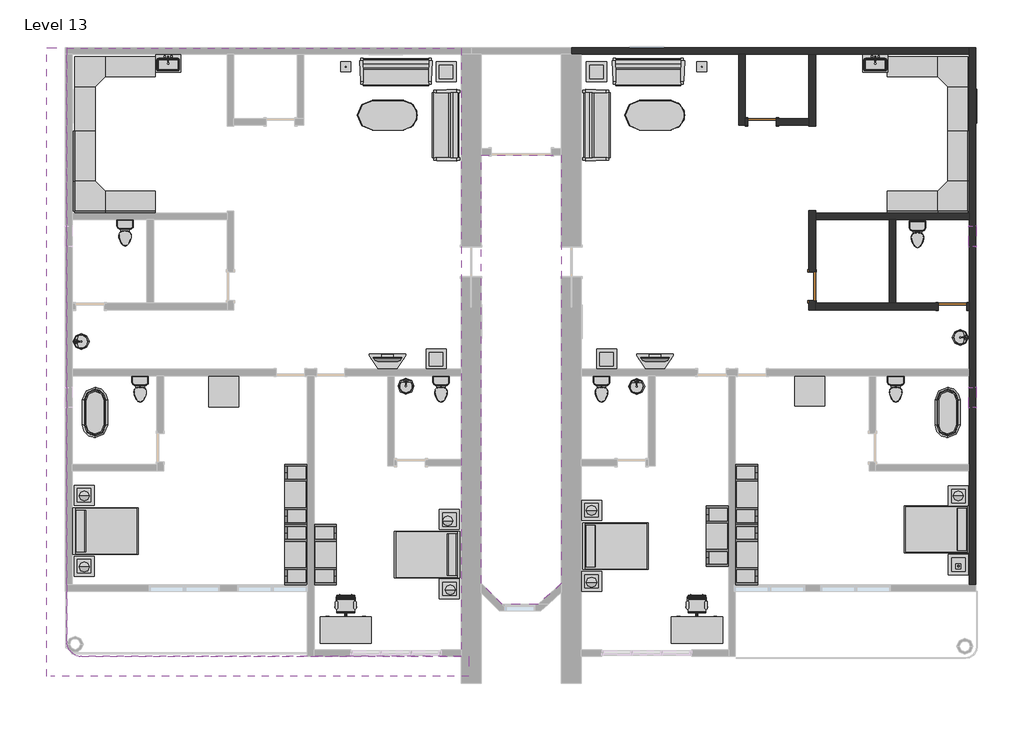
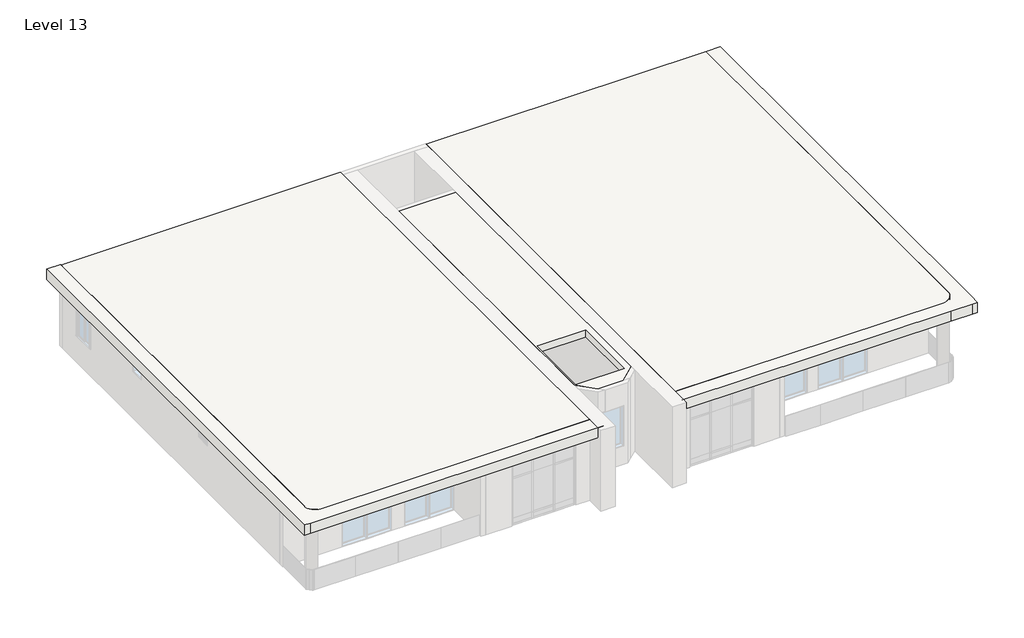
# One storey, part 3 of 3: 42 furniture elements, 14 flow terminals, 10 light fixtures, 9 walls, 3 doors, 3 slabs, 3 windows.
# Revit data of these elements (continued)
# Elements 38, 39 (IfcFurniture, "TV - Flat Screen : 32\"")
#   Stand = yes
#   Phase Created = New Construction
#   Materials on its faces: "TV - Black", "TV - Glass", "TV - Screen"
# Elements 40, 41 (IfcFurniture, "TV Stand : TV Stand")
#   Phase Created = New Construction
#   Materials on its faces: "Melamine - Gray", "Glass - Shelves"
# Elements 42, 43, 44, 45, 46, 47, 48, 49, 50, 51, 52, 53 (IfcFurniture, "Table-Coffee : 24\" x 24\" x 24\"")
#   Phase Created = New Construction
#   Materials on its faces: "Glass - Clear, Grey"
# Elements 54, 55 (IfcFurniture, "Table-Dining Oval : 36\" x 72\"")
#   Phase Created = New Construction
#   Materials on its faces: "Steel, Chrome Plated", "Glass - Clear, Grey"
# Elements 56, 57 (IfcFurniture, "Table-Rectangular : 36\" x 36\"")
#   Phase Created = New Construction
#   Materials on its faces: "Birch"
# Elements 58, 59 (IfcFurniture, "Work Station Cubicle : 96\" x 96\"")
#   Phase Created = New Construction
#   Materials on its faces: "Textile - Light Gray", "Laminate, Ivory, Matte"
# Element 60 (IfcLightFixture, "100W - 120V")
#   Mark = "144"
#   Phase Created = New Construction
#   Materials on its faces: "Steel, Chrome Plated", "Glass, Frosted"
# Element 61 (IfcLightFixture, "100W - 120V")
#   Mark = "145"
#   Phase Created = New Construction
#   Materials on its faces: "Steel, Chrome Plated", "Glass, Frosted"
# Element 62 (IfcLightFixture, "Table Lamp - Hemispheric : 60W - 120V")
#   Mark = "146"
#   Phase Created = New Construction
#   Materials on its faces: "Steel, Chrome Plated", "Glass, Frosted", "Birch"
# Element 63 (IfcLightFixture, "Table Lamp - Hemispheric : 60W - 120V")
#   Mark = "147"
#   Phase Created = New Construction
#   Materials on its faces: "Steel, Chrome Plated", "Glass, Frosted", "Birch"
# Element 64 (IfcLightFixture, "Table Lamp - Hemispheric : 60W - 120V")
#   Mark = "148"
#   Phase Created = New Construction
#   Materials on its faces: "Steel, Chrome Plated", "Glass, Frosted", "Birch"
# Element 65 (IfcLightFixture, "Table Lamp - Hemispheric : 60W - 120V")
#   Mark = "149"
#   Phase Created = New Construction
#   Materials on its faces: "Steel, Chrome Plated", "Glass, Frosted", "Birch"
# Element 66 (IfcLightFixture, "Table Lamp - Hemispheric : 60W - 120V")
#   Mark = "150"
#   Phase Created = New Construction
#   Materials on its faces: "Steel, Chrome Plated", "Glass, Frosted", "Birch"
# Element 67 (IfcLightFixture, "Table Lamp - Hemispheric : 60W - 120V")
#   Mark = "151"
#   Phase Created = New Construction
#   Materials on its faces: "Steel, Chrome Plated", "Glass, Frosted", "Birch"
# Element 68 (IfcLightFixture, "Table Lamp - Hemispheric : 60W - 120V")
#   Mark = "152"
#   Phase Created = New Construction
#   Materials on its faces: "Steel, Chrome Plated", "Glass, Frosted", "Birch"
# Element 69 (IfcLightFixture, "Table Lamp - Hemispheric : 60W - 120V")
#   Mark = "153"
#   Phase Created = New Construction
#   Materials on its faces: "Steel, Chrome Plated", "Glass, Frosted", "Birch"
# Element 70 (IfcSlab, "Generic - 1.5' white 2")
#   built-in parameter 1001955 = 3.14159 (stored number, unit not read)
#   Height Offset From Level = 12' - 0"
#   Phase Created = New Construction
#   Materials on its faces: "Door - Frame"
# Element 71 (IfcSlab, "Generic - 12\" cream")
#   Height Offset From Level = 12' - 0"
#   Phase Created = New Construction
#   Materials on its faces: "Parking Stripe"
# Element 72 (IfcSlab, "Generic - 12\" white")
#   Height Offset From Level = 12' - 0"
#   Phase Created = New Construction
#   Materials on its faces: "Door - Frame"
# Elements 73, 74, 75, 76, 77, 78, 79, 80 (IfcWall, "Generic - 8\" cream")
#   Top Offset = 0' - 0"
#   Base Offset = 0' - 0"
#   Unconnected Height = 10' - 0"
#   wall height = 10' - 0"
#   Phase Created = New Construction
#   Base Constraint = Level 13
#   Materials on its faces: "Parking Stripe"
# Element 81 (IfcWall, "Generic - 8\" white")
#   Top Offset = 0' - 0"
#   Base Offset = 0' - 0"
#   Unconnected Height = 10' - 0"
#   wall height = 10' - 0"
#   Phase Created = New Construction
#   Base Constraint = Level 13
#   Materials on its faces: "Door - Frame", "Parking Stripe"
# Element 82 (IfcWindow, "Louvers with Trim : 24\" x 24\"")
#   Mark = "281"
#   Phase Created = New Construction
#   Materials on its faces: "Glass", "Iron, Ductile"
# Element 83 (IfcWindow, "Louvers with Trim : 24\" x 24\"")
#   Mark = "282"
#   Phase Created = New Construction
#   Materials on its faces: "Glass", "Iron, Ductile"
# Element 84 (IfcWindow, "Slider with Trim : 36\" x 48\"")
#   Mark = "278"
#   Phase Created = New Construction
#   Materials on its faces: "Iron, Ductile", "Glass"
# Materials
#   "Wood - Birch - Solid Stained Light Low Gloss": class "Wood", colour RGB 210 159 95, transparency 0, Cost = 0
#   "Paint - Sienna": colour RGB 118 70 51, transparency 0, Cost = 0
#   "Steel, Polished": class "Metal", colour RGB 57 57 57, transparency 0, Description = "Polished steel", Cost = 0
#   "Porcelain, Linen": class "Ceramic", colour RGB 249 239 230, transparency 0, Description = "Porcelain, linen", Cost = 0
#   "Laminate, Linen, Matte": class "Plastic", colour RGB 249 239 230, transparency 0, Description = "Plastic Laminate - Linen, Matte", Cost = 0
#   "Porcelain, Ivory": class "Ceramic", colour RGB 247 247 239, transparency 0, Description = "Porcelain, ivory", Cost = 0
#   "Laminate, Ivory, Matte": class "Plastic", colour RGB 247 247 239, transparency 0, Description = "Plastic Laminate - Ivory, Matte", Cost = 0
#   "Birch": class "Wood", colour RGB 224 178 126, transparency 0, Description = "Betula Alleghaniensis", Cost = 0
#   "Linen, White": class "Textile", colour RGB 247 247 239, transparency 0, Description = "Linen, white", Cost = 0
#   "Plastic, Opaque Black": class "Plastic", colour RGB 0 0 0, transparency 0.7, Description = "Plastic, generic, opaque black", Cost = 0
#   "Textile - Slate Blue": class "Fabric", colour RGB 98 102 118, transparency 0
#   "Steel, Chrome Plated": class "Metal", colour RGB 17 17 17, transparency 0, Description = "Chromiuim plated steel", Cost = 0
#   "Cherry": class "Wood", colour RGB 226 177 128, transparency 0, Description = "Prunus Serotina", Cost = 0
#   "Linen, Beige": class "Textile", colour RGB 249 239 230, transparency 0, Description = "Linen, beige", Cost = 0
#   "Melamine - Gray": class "Wood", colour RGB 49 49 49, transparency 0
#   "Glass - Clear, Grey": class "Glass", colour RGB 252 255 255, transparency 0.64
#   "Textile - Light Gray": class "Fabric", colour RGB 204 204 204, transparency 0
#   "Glass, Frosted": class "Glass", colour RGB 250 244 225, transparency 0.55, Description = "physical material", Cost = 0
#   "Door - Frame": colour RGB 118 70 51, transparency 0, Cost = 0
#   "Parking Stripe": class "Paint", colour RGB 250 250 91, transparency 0, Cost = 0
#   "Iron, Ductile": class "Metal", colour RGB 0 0 0, transparency 0, Description = "Ductile cast iron", Cost = 0
#   "Glass": class "Glass", colour RGB 0 128 192, transparency 0.75, Description = "Soda Lime Glass", Cost = 0
#   "TV - Black": colour RGB 49 49 49, transparency 0
#   "TV - Glass": colour RGB 157 157 157, transparency 0.9
#   "TV - Screen": colour RGB 0 0 0, transparency 0
#   "Glass - Shelves": class "Glass", colour RGB 167 167 167, transparency 0.9
